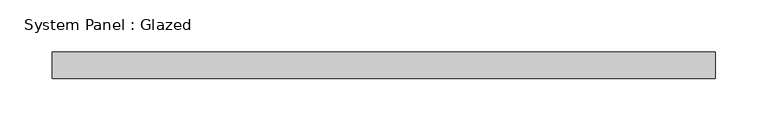
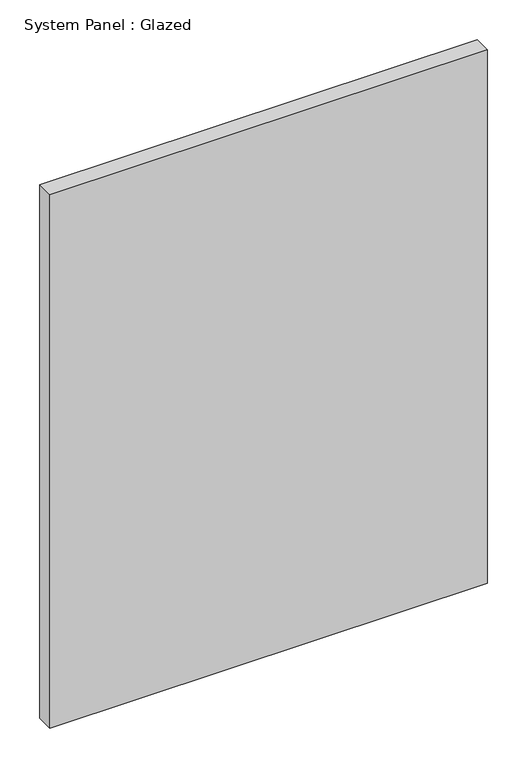
"""IFC4 building model written with IfcOpenShell, lengths in millimetres: plate geometry, System Panel : Glazed."""

from ifc_helpers import new_model, si_unit, origin, origin_with_axes, place, context, project, spatial, polyline, outline, extrude, source, transform, mapped, element, save


def system_panel_glazed_1d091053(model_context):
    return source(origin(), model_context, "Body", "SweptSolid", [
        extrude(outline(polyline([(317.5, 19.05), (-317.5, 19.05), (-317.5, 44.45), (317.5, 44.45), (317.5, 19.05)])), origin_with_axes(), (0.0, 0.0, 1.0), 819.15),
    ])


if __name__ == "__main__":
    model = new_model("IFC4")
    model_context = context("Model", 3, world=origin())
    ifc_project = project(units=[si_unit("LENGTHUNIT", "METRE", prefix="MILLI")], contexts=[model_context])
    site = spatial("IfcSite", under=ifc_project)
    building = spatial("IfcBuilding", under=site)
    placement = place(None, origin())
    system_panel_glazed_shape = system_panel_glazed_1d091053(model_context)
    element("IfcPlate", 1, ObjectType="System Panel : Glazed", at=placement, inside=building, context=model_context, shape_type="MappedRepresentation", body=[
        mapped(system_panel_glazed_shape, transform((0.0, 0.0, 0.0), x_axis=(1.0, 0.0, 0.0), y_axis=(0.0, 1.0, 0.0), z_axis=(0.0, 0.0, 1.0))),
    ])
    save(model, "model.ifc")

# Revit data of these elements
# Type "System Panel : Glazed"
#   Construction Type Id = "GSP4R"
#   Analytic Construction = "1/8 in Pilkington single glazing"
#   Visual Light Transmittance = 0.9
#   Solar Heat Gain Coefficient = 0.86
#   Heat Transfer Coefficient (U) = 1.18115 BTU/(h·ft²·°F)
# Element 1 (IfcPlate, "System Panel : Glazed")
#   Materials on its faces: "Glass"
# Materials
#   "Glass": class "Glass", colour RGB 0 128 192, transparency 0.75, Description = "Soda Lime Glass", Cost = 0
